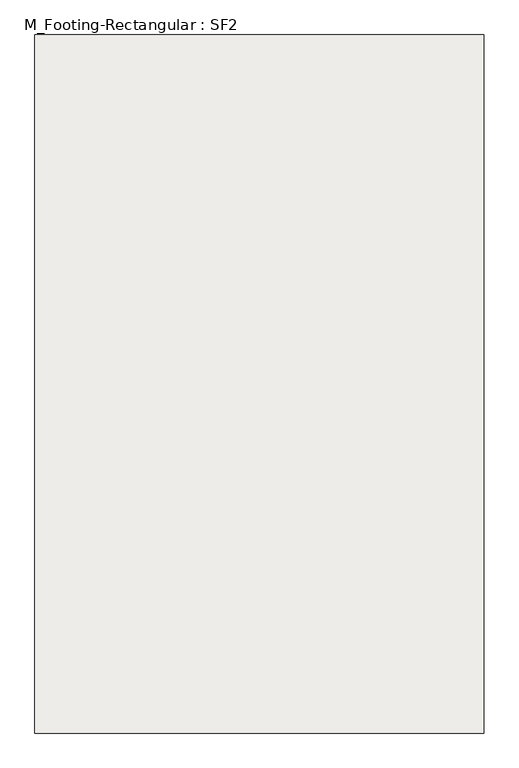
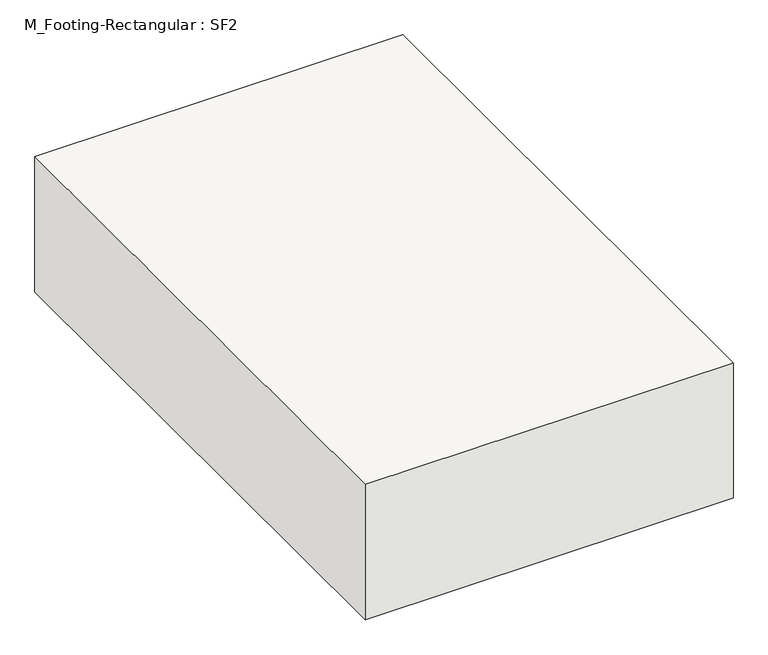
"""IFC4 building model written with IfcOpenShell, lengths in millimetres: slab geometry, M_Footing-Rectangular : SF2."""

from ifc_helpers import new_model, si_unit, frame, origin, place, context, project, spatial, polyline, outline, extrude, source, transform, mapped, element, save


def m_footing_rectangular_sf2_5cd490c0(model_context):
    return source(origin(), model_context, "Body", "SweptSolid", [
        extrude(outline(polyline([(685.8, 1066.8), (685.8, -1066.8), (-685.8, -1066.8), (-685.8, 1066.8), (685.8, 1066.8)])), frame((0.0, 0.0, -533.4), z_axis=(0.0, 0.0, 1.0), x_axis=(1.0, 0.0, 0.0)), (0.0, 0.0, 1.0), 533.4),
    ])


if __name__ == "__main__":
    model = new_model("IFC4")
    model_context = context("Model", 3, world=origin())
    ifc_project = project(units=[si_unit("LENGTHUNIT", "METRE", prefix="MILLI")], contexts=[model_context])
    site = spatial("IfcSite", under=ifc_project)
    building = spatial("IfcBuilding", under=site)
    placement = place(None, origin())
    m_footing_rectangular_sf2_shape = m_footing_rectangular_sf2_5cd490c0(model_context)
    element("IfcSlab", 1, ObjectType="M_Footing-Rectangular : SF2", at=placement, inside=building, context=model_context, shape_type="MappedRepresentation", body=[
        mapped(m_footing_rectangular_sf2_shape, transform((0.0, 0.0, 0.0), x_axis=(1.0, 0.0, 0.0), y_axis=(0.0, 1.0, 0.0), z_axis=(0.0, 0.0, 1.0))),
    ])
    save(model, "model.ifc")

# Revit data of these elements
# Type "M_Footing-Rectangular : SF2"
#   Width = 1371.6 mm
#   Length = 2133.6 mm
#   Foundation Thickness = 533.4 mm
#   Structural Material [instance default] = Concrete, Cast-in-Place gray
#   Assembly Code = ""
# Element 1 (IfcSlab, "M_Footing-Rectangular : SF2")
#   Materials on its faces: "Concrete, Cast-in-Place gray"
# Materials
#   "Concrete, Cast-in-Place gray": class "Concrete", colour RGB 192 192 192, transparency 0, Description = "Cast-in-place concrete", Cost = 0
